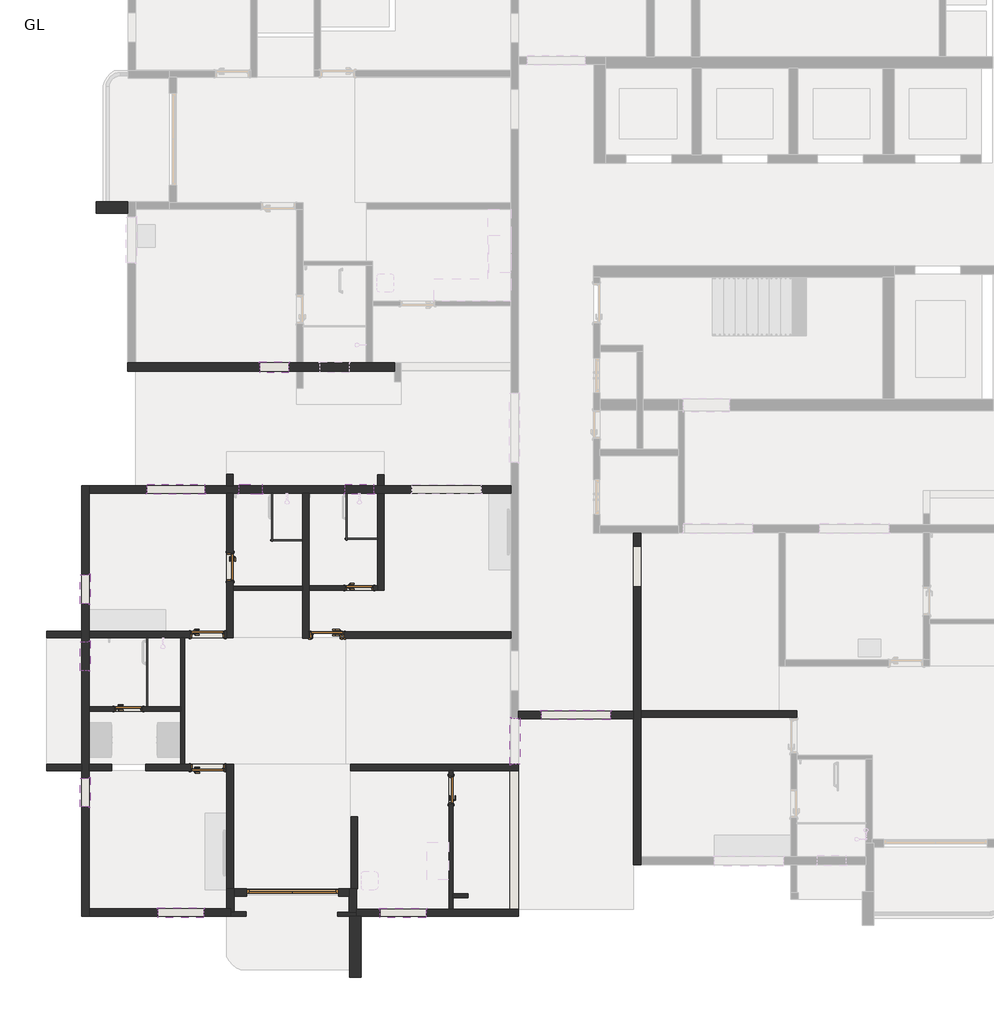
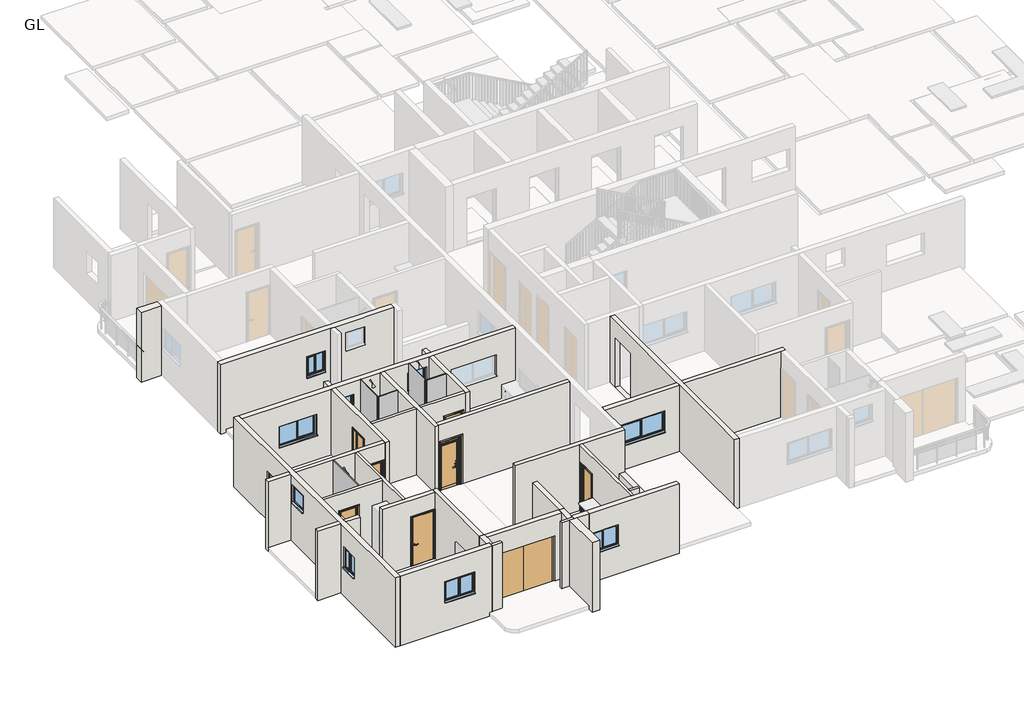
# One storey, part 1 of 14: 36 walls, 11 windows, 9 doors, 5 plates.
# Revit data of these elements (continued)
# Type "Windows_Dbl_Plain : 4'" (continued)
#   Heat Transfer Coefficient (U) = 3.6886 W/(m²·K)
#   Glazing Thickness = 0.07874 ft
#   FrameOffset - External = 0.164042 ft
#   Frame Depth = 0.213255 ft
#   Default Head Height = 6.922572 ft
#   Cill Depth = 0.287073 ft
#   Cavity Closer Width = 0.164042 ft
#   Cavity Closer Offset from Ext = 0.336286 ft
#   Cavity Closer Depth = 0.278871 ft
#   Vis - Cavity Closers = yes
#   Define Thermal Properties by = 1
#   Material Trim = Window Frame
#   Material Glass = Glass
#   Material Frame = Window Frame
#   Wall Closure = (empty or 0)
# Type "Windows_Dbl_Plain : 5'"
#   Type Mark = "58"
#   Operation = "DoublePanelVertical"
#   Construction Type Id = "GSP4R"
#   Manufacturer = "Revit"
#   Keynote = "L10"
#   Analytic Construction = "1/8 in Pilkington single glazing"
#   Wrap Layers (Ext) from Ext = 0.336286 ft
#   Wrap Layers (Int) from Ext = 0.582349 ft
#   Window Board Projection = 0.082021 ft
#   Window Board Extension = 0.082021 ft
#   Visual Light Transmittance = 0.9
#   Solar Heat Gain Coefficient = 0.78
#   Rough Width = 5.0 ft
#   Rough Height = 2.985564 ft
#   Height = 2.985564 ft
#   Width = 5.0 ft
#   Heat Transfer Coefficient (U) = 3.6886 W/(m²·K)
#   Glazing Thickness = 0.07874 ft
#   FrameOffset - External = 0.164042 ft
#   Frame Depth = 0.213255 ft
#   Default Head Height = 6.922572 ft
#   Cill Depth = 0.287073 ft
#   Cavity Closer Width = 0.164042 ft
#   Cavity Closer Offset from Ext = 0.336286 ft
#   Cavity Closer Depth = 0.278871 ft
#   Vis - Cavity Closers = yes
#   Define Thermal Properties by = 1
#   Material Trim = Window Frame
#   Material Glass = Glass
#   Material Frame = Window Frame
#   Wall Closure = (empty or 0)
# Type "Windows_Dbl_Plain : 6'"
#   Type Mark = "62"
#   Operation = "DoublePanelVertical"
#   Construction Type Id = "GSP4R"
#   Manufacturer = "Revit"
#   Keynote = "L10"
#   Analytic Construction = "1/8 in Pilkington single glazing"
#   Wrap Layers (Ext) from Ext = 0.336286 ft
#   Wrap Layers (Int) from Ext = 0.582349 ft
#   Window Board Projection = 0.082021 ft
#   Window Board Extension = 0.082021 ft
#   Visual Light Transmittance = 0.9
#   Solar Heat Gain Coefficient = 0.78
#   Rough Width = 6.0 ft
#   Rough Height = 2.985564 ft
#   Height = 2.985564 ft
#   Width = 6.0 ft
#   Heat Transfer Coefficient (U) = 3.6886 W/(m²·K)
#   Glazing Thickness = 0.07874 ft
#   FrameOffset - External = 0.164042 ft
#   Frame Depth = 0.213255 ft
#   Default Head Height = 6.922572 ft
#   Cill Depth = 0.287073 ft
#   Cavity Closer Width = 0.164042 ft
#   Cavity Closer Offset from Ext = 0.336286 ft
#   Cavity Closer Depth = 0.278871 ft
#   Vis - Cavity Closers = yes
#   Define Thermal Properties by = 1
#   Material Trim = Window Frame
#   Material Glass = Glass
#   Material Frame = Window Frame
#   Wall Closure = (empty or 0)
# Type "Windows_Sgl_Plain : 2'"
#   Type Mark = "60"
#   Operation = "SinglePanel"
#   Construction Type Id = "SGL"
#   Manufacturer = "Revit"
#   Keynote = "L10"
#   Analytic Construction = "Large single-glazed windows"
#   Wrap Layers (Ext) from Ext = 0.336286 ft
#   Wrap Layers (Int) from Ext = 0.582349 ft
#   Window Board Projection = 0.082021 ft
#   Window Board Extension = 0.082021 ft
#   Visual Light Transmittance = 0.9
#   Solar Heat Gain Coefficient = 0.86
#   Rough Width = 2.0 ft
#   Rough Height = 2.0 ft
#   Height = 2.0 ft
#   Width = 2.0 ft
#   Heat Transfer Coefficient (U) = 5.5617 W/(m²·K)
#   Glazing Thickness = 0.07874 ft
#   FrameOffset - External = 0.164042 ft
#   Frame Depth = 0.213255 ft
#   Default Head Height = 6.922572 ft
#   Cill Depth = 0.287073 ft
#   Cavity Closer Width = 0.164042 ft
#   Cavity Closer Offset from Ext = 0.336286 ft
#   Cavity Closer Depth = 0.278871 ft
#   Vis - Cavity Closers = yes
#   Define Thermal Properties by = 1
#   Material Trim = Window Frame
#   Material Glass = Glass
#   Material Frame = Window Frame
#   Wall Closure = (empty or 0)
# Type "Windows_Sgl_Plain : 2.5'"
#   Type Mark = "61"
#   Operation = "SinglePanel"
#   Construction Type Id = "SGL"
#   Manufacturer = "Revit"
#   Keynote = "L10"
#   Analytic Construction = "Large single-glazed windows"
#   Wrap Layers (Ext) from Ext = 0.336286 ft
#   Wrap Layers (Int) from Ext = 0.582349 ft
#   Window Board Projection = 0.082021 ft
#   Window Board Extension = 0.082021 ft
#   Visual Light Transmittance = 0.9
#   Solar Heat Gain Coefficient = 0.86
#   Rough Width = 2.5 ft
#   Rough Height = 2.5 ft
#   Height = 2.5 ft
#   Width = 2.5 ft
#   Heat Transfer Coefficient (U) = 5.5617 W/(m²·K)
#   Glazing Thickness = 0.07874 ft
#   FrameOffset - External = 0.164042 ft
#   Frame Depth = 0.213255 ft
#   Default Head Height = 6.922572 ft
#   Cill Depth = 0.287073 ft
#   Cavity Closer Width = 0.164042 ft
#   Cavity Closer Offset from Ext = 0.336286 ft
#   Cavity Closer Depth = 0.278871 ft
#   Vis - Cavity Closers = yes
#   Define Thermal Properties by = 1
#   Material Trim = Window Frame
#   Material Glass = Glass
#   Material Frame = Window Frame
#   Wall Closure = (empty or 0)
# Element 1 (IfcDoor, "Doors_Concept_ExtDbl : 8'")
#   Phase Created = New Construction
#   Materials on its faces: "Concept", "Door - Glazing"
# Elements 2, 3, 4, 5 (IfcDoor, "Doors_IntSgl : 2.5' DOOR")
#   Phase Created = New Construction
#   Materials on its faces: "Door - Architrave", "Door - Handle", "Door - Frame/Mullion (1)", "Door - Panel"
# Elements 6, 7, 8 (IfcDoor, "Doors_IntSgl : 3' DOOR")
#   Phase Created = New Construction
#   Materials on its faces: "Door - Architrave", "Door - Handle", "Door - Frame/Mullion (1)", "Door - Panel"
# Element 9 (IfcDoor, "Doors_IntSgl : 810x2110mm")
#   Phase Created = New Construction
#   Materials on its faces: "Door - Architrave", "Door - Handle", "Door - Frame/Mullion (1)", "Door - Panel"
# Elements 10, 11, 12, 13, 14 (IfcPlate, "System Panel : Glazed")
#   Phase Created = New Construction
#   Materials on its faces: "Glass"
# Elements 15, 16, 17, 18, 19, 20, 21, 22, 23, 24, 25, 26, 27, 28 (IfcWall, "W2")
#   Top Offset = 0.0 ft
#   Base Offset = 0.0 ft
#   wall height = 9.84252 ft
#   Phase Created = New Construction
#   Base Constraint = GL
#   Top Constraint = FFL
#   Materials on its faces: "Brick, Common"
# Elements 29, 30, 31, 32, 33, 34, 35, 36 (IfcWall, "W3")
#   Top Offset = 0.0 ft
#   Base Offset = 0.0 ft
#   wall height = 9.84252 ft
#   Phase Created = New Construction
#   Base Constraint = GL
#   Top Constraint = FFL
#   Materials on its faces: "Brick, Common"
# Elements 37, 38 (IfcWall, "W4")
#   Top Offset = 0.0 ft
#   Base Offset = 0.0 ft
#   wall height = 9.84252 ft
#   Phase Created = New Construction
#   Base Constraint = GL
#   Top Constraint = FFL
#   Materials on its faces: "Brick, Common"
# Element 39 (IfcWall, "W5")
#   Top Offset = -6.0 ft
#   Base Offset = 0.0 ft
#   wall height = 3.84252 ft
#   Phase Created = New Construction
#   Base Constraint = GL
#   Top Constraint = FFL
#   Materials on its faces: "Brick, Common"
# Element 40 (IfcWall, "W5")
#   Top Offset = 0.0 ft
#   Base Offset = 0.0 ft
#   wall height = 9.84252 ft
#   Phase Created = New Construction
#   Base Constraint = GL
#   Top Constraint = FFL
#   Materials on its faces: "Brick, Common"
# Elements 41, 42, 43, 44, 45, 46, 47, 48, 49, 50 (IfcWall, "WALL 1")
#   Top Offset = 0.0 ft
#   Base Offset = 0.0 ft
#   wall height = 9.84252 ft
#   Phase Created = New Construction
#   Base Constraint = GL
#   Top Constraint = FFL
#   Materials on its faces: "Brick, Common"
# Element 51 (IfcWindow, "Windows_Dbl_Plain : 2.5'")
#   Mark = "2"
#   Phase Created = New Construction
#   Materials on its faces: "Window Frame", "Glass"
# Element 52 (IfcWindow, "Windows_Dbl_Plain : 2.5'")
#   Mark = "4"
#   Phase Created = New Construction
#   Materials on its faces: "Window Frame", "Glass"
# Element 53 (IfcWindow, "Windows_Dbl_Plain : 2.5'")
#   Mark = "59"
#   Phase Created = New Construction
#   Materials on its faces: "Window Frame", "Glass"
# Element 54 (IfcWindow, "Windows_Dbl_Plain : 4'")
#   Mark = "1"
#   Phase Created = New Construction
#   Materials on its faces: "Window Frame", "Glass"
# Element 55 (IfcWindow, "Windows_Dbl_Plain : 4'")
#   Mark = "11"
#   Phase Created = New Construction
#   Materials on its faces: "Window Frame", "Glass"
# Element 56 (IfcWindow, "Windows_Dbl_Plain : 4'")
#   Mark = "12"
#   Phase Created = New Construction
#   Materials on its faces: "Window Frame", "Glass"
# Element 57 (IfcWindow, "Windows_Dbl_Plain : 5'")
#   Mark = "5"
#   Phase Created = New Construction
#   Materials on its faces: "Window Frame", "Glass"
# Element 58 (IfcWindow, "Windows_Dbl_Plain : 6'")
#   Mark = "13"
#   Phase Created = New Construction
#   Materials on its faces: "Window Frame", "Glass"
# Element 59 (IfcWindow, "Windows_Sgl_Plain : 2'")
#   Mark = "7"
#   Phase Created = New Construction
#   Materials on its faces: "Window Frame", "Glass"
# Element 60 (IfcWindow, "Windows_Sgl_Plain : 2.5'")
#   Mark = "3"
#   Phase Created = New Construction
#   Materials on its faces: "Window Frame", "Glass"
# Element 61 (IfcWindow, "Windows_Sgl_Plain : 2.5'")
#   Mark = "8"
#   Phase Created = New Construction
#   Materials on its faces: "Window Frame", "Glass"
# Materials
#   "Door - Glazing": colour RGB 0 0 255, transparency 0.75
#   "Concept": colour RGB 128 128 255, transparency 0.5
#   "Door - Handle": colour RGB 0 0 0, transparency 0, Keynote = "P21", Cost = 0
#   "Door - Frame/Mullion (1)": class "Wood", colour RGB 212 179 113, transparency 0, Keynote = "L20", Cost = 0
#   "Door - Panel": class "Wood", colour RGB 210 159 95, transparency 0, Keynote = "L20", Cost = 0
#   "Door - Architrave": class "Wood", colour RGB 154 90 5, transparency 0, Keynote = "P20", Cost = 0
#   "Brick, Common": class "Masonry", colour RGB 170 100 105, transparency 0, Description = "Common brick", Cost = 0
#   "Window Frame": colour RGB 249 249 249, transparency 0, Keynote = "L10", Cost = 0
#   "Glass": class "Glass", colour RGB 0 128 192, transparency 0.9, Description = "Soda Lime Glass", Cost = 0
# Room, not placed, phase "New Construction", upper offset 0.0 ft, lower offset 0.0 ft
#   Number = "1"
#   Name = "Room"
